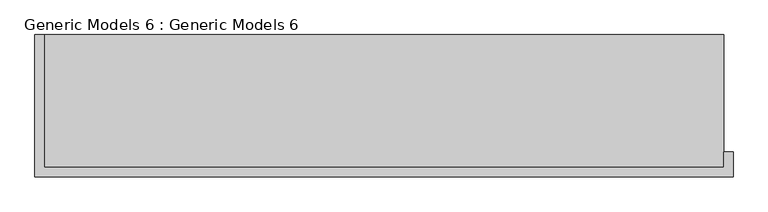
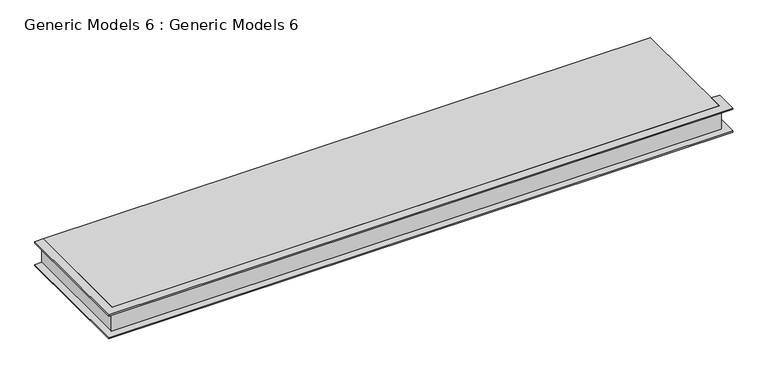
"""IFC4 building model written with IfcOpenShell, lengths in millimetres: proxy geometry, Generic Models 6 : Generic Models 6."""

from ifc_helpers import new_model, si_unit, frame, origin, place, context, project, spatial, polyline, outline, extrude, faceted_brep, source, transform, mapped, element, save


def generic_models_6_generic_models_6_4d21afab(model_context):
    return source(origin(), model_context, "Body", "SolidModel", [
        faceted_brep([(8173.5271331, -12915.5643494, 7924.8), (8173.5271331, -12915.5643494, 7912.1), (8110.0271331, -12915.5643494, 7912.1), (8110.0271331, -12915.5643494, 7708.9), (8173.5271331, -12915.5643494, 7708.9), (8173.5271331, -12915.5643494, 7696.2), (8097.3271331, -12915.5643494, 7696.2), (8097.3271331, -12915.5643494, 7924.8), (8173.5271331, -13118.7643494, 7924.8), (8173.5271331, -13118.7643494, 7912.1), (2572.8271331, -13118.7643494, 7912.1), (2572.8271331, -11975.7643494, 7912.1), (2636.3271331, -11975.7643494, 7912.1), (2636.3271331, -13055.2643494, 7912.1), (8110.0271331, -13055.2643494, 7912.1), (8110.0271331, -13055.2643494, 7708.9), (2636.3271331, -13055.2643494, 7708.9), (2636.3271331, -11975.7643494, 7708.9), (2572.8271331, -11975.7643494, 7708.9), (2572.8271331, -13118.7643494, 7708.9), (8173.5271331, -13118.7643494, 7708.9), (8173.5271331, -13118.7643494, 7696.2), (2572.8271331, -13118.7643494, 7696.2), (2572.8271331, -11975.7643494, 7696.2), (2649.0271331, -11975.7643494, 7696.2), (2649.0271331, -13042.5643494, 7696.2), (8097.3271331, -13042.5643494, 7696.2), (8097.3271331, -13042.5643494, 7924.8), (2649.0271331, -13042.5643494, 7924.8), (2649.0271331, -11975.7643494, 7924.8), (2572.8271331, -11975.7643494, 7924.8), (2572.8271331, -13118.7643494, 7924.8)], [[[0, 1, 2, 3, 4, 5, 6, 7]], [[1, 0, 8, 9]], [[2, 1, 9, 10, 11, 12, 13, 14]], [[3, 2, 14, 15]], [[4, 3, 15, 16, 17, 18, 19, 20]], [[5, 4, 20, 21]], [[6, 5, 21, 22, 23, 24, 25, 26]], [[7, 6, 26, 27]], [[0, 7, 27, 28, 29, 30, 31, 8]], [[9, 8, 31, 10]], [[15, 14, 13, 16]], [[21, 20, 19, 22]], [[27, 26, 25, 28]], [[30, 29, 24, 23, 18, 17, 12, 11]], [[10, 31, 30, 11]], [[16, 13, 12, 17]], [[22, 19, 18, 23]], [[28, 25, 24, 29]]]),
        extrude(outline(polyline([(8097.3271331, -13042.5643494), (2649.0271331, -13042.5643494), (2649.0271331, -11975.7643494), (8097.3271331, -11975.7643494), (8097.3271331, -13042.5643494)])), frame((0.0, 0.0, 7696.2), z_axis=(0.0, 0.0, 1.0), x_axis=(1.0, 0.0, 0.0)), (0.0, 0.0, 1.0), 228.6),
    ])


if __name__ == "__main__":
    model = new_model("IFC4")
    model_context = context("Model", 3, world=origin())
    ifc_project = project(units=[si_unit("LENGTHUNIT", "METRE", prefix="MILLI")], contexts=[model_context])
    site = spatial("IfcSite", under=ifc_project)
    building = spatial("IfcBuilding", under=site)
    placement = place(None, origin())
    generic_models_6_generic_models_6_shape = generic_models_6_generic_models_6_4d21afab(model_context)
    element("IfcBuildingElementProxy", 1, Name="Generic Models 6 : Generic Models 6", ObjectType="Generic Models 6 : Generic Models 6", at=placement, inside=building, context=model_context, shape_type="MappedRepresentation", body=[
        mapped(generic_models_6_generic_models_6_shape, transform((0.0, 0.0, 0.0), x_axis=(1.0, 0.0, 0.0), y_axis=(0.0, 1.0, 0.0), z_axis=(0.0, 0.0, 1.0))),
    ])
    save(model, "model.ifc")
